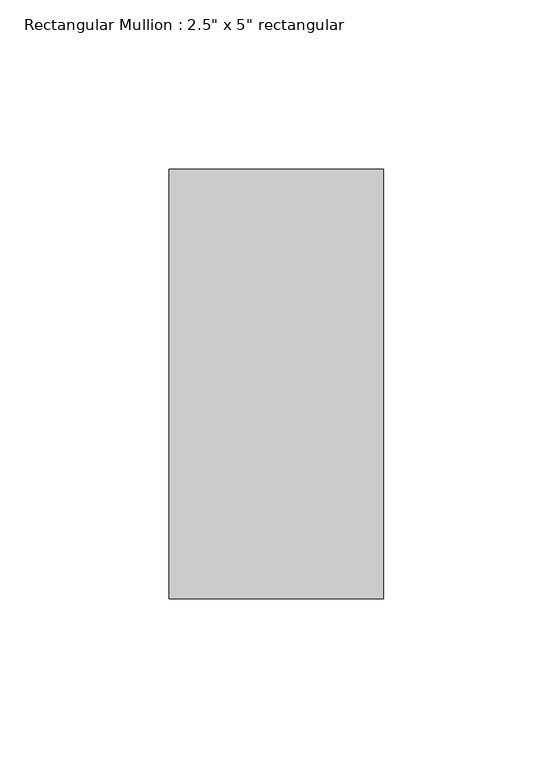
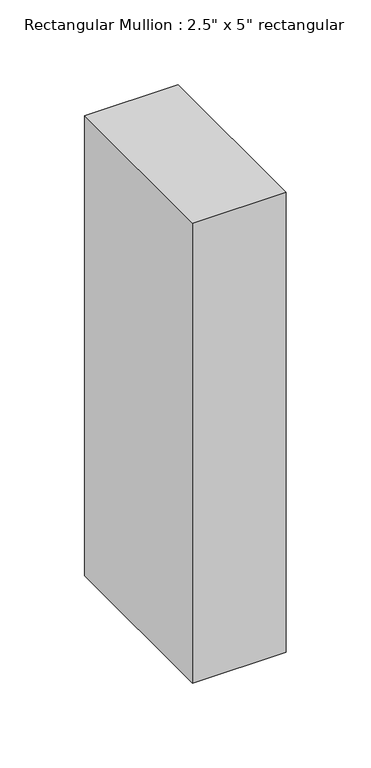
"""IFC4 building model written with IfcOpenShell, lengths in millimetres: member geometry."""

from ifc_helpers import new_model, si_unit, frame, origin, place, context, project, spatial, polyline, outline, extrude, source, transform, mapped, element, save


def member_1c9aee36(model_context):
    return source(origin(), model_context, "Body", "SweptSolid", [
        extrude(outline(polyline([(31.75, 63.5), (31.75, -63.5), (-31.75, -63.5), (-31.75, 63.5), (31.75, 63.5)])), frame((0.0, 0.0, -330.4597418), z_axis=(0.0, 0.0, 1.0), x_axis=(1.0, 0.0, 0.0)), (0.0, 0.0, 1.0), 330.4597418),
    ])


if __name__ == "__main__":
    model = new_model("IFC4")
    model_context = context("Model", 3, world=origin())
    ifc_project = project(units=[si_unit("LENGTHUNIT", "METRE", prefix="MILLI")], contexts=[model_context])
    site = spatial("IfcSite", under=ifc_project)
    building = spatial("IfcBuilding", under=site)
    placement = place(None, origin())
    member_shape = member_1c9aee36(model_context)
    element("IfcMember", 1, ObjectType="Rectangular Mullion : 2.5\" x 5\" rectangular", at=placement, inside=building, context=model_context, shape_type="MappedRepresentation", body=[
        mapped(member_shape, transform((0.0, 0.0, 0.0), x_axis=(1.0, 0.0, 0.0), y_axis=(0.0, 1.0, 0.0), z_axis=(0.0, 0.0, 1.0))),
    ])
    save(model, "model.ifc")

# Revit data of these elements
# Type "Rectangular Mullion : 2.5\" x 5\" rectangular"
#   built-in parameter 1007304 = 0.416667 (stored number, unit not read)
#   built-in parameter 1007301 = 0.104167 (stored number, unit not read)
#   built-in parameter 1007300 = 0.104167 (stored number, unit not read)
